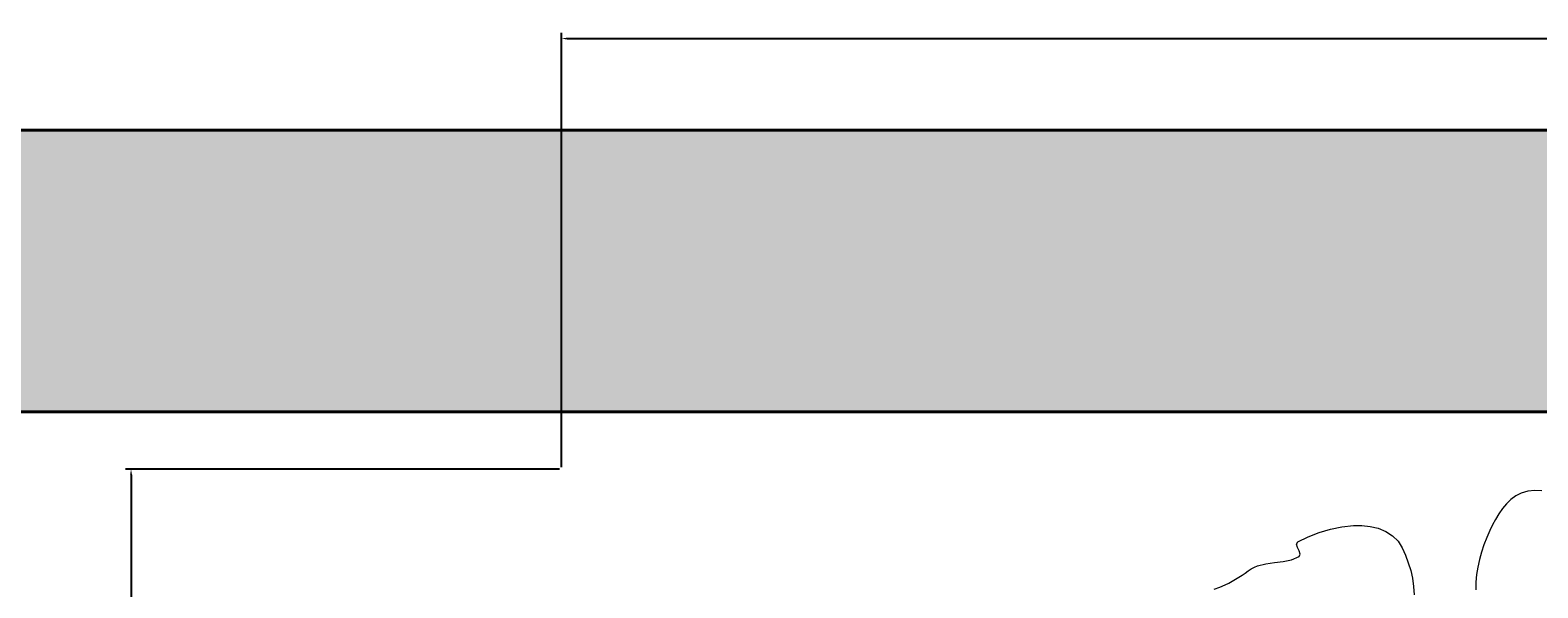
# Model space of a CAD drawing. Units: inches. Extents: x 1441 to 2460, y 1648 to 2683.
# Tile 27 of 35: x 1792 to 1840, y 2284 to 2302. Entities that reach past the tile are written whole.
import ezdxf

# ---------------------------------------------------------------- set-up
doc = ezdxf.new("R2010")
doc.units = ezdxf.units.IN
for name, color, linetype, lineweight in [('A-ANNO-DIMS', 2, 'Continuous', 18), ('A-FURN', 8, 'Continuous', 15), ('A-WALL', 7, 'Continuous', 40)]:
    doc.layers.add(name, color=color, linetype=linetype, lineweight=lineweight)
doc.layers.add('A-WALL-PATT', color=251, linetype='Continuous', lineweight=13, true_color=0x636466)
doc.styles.get("Standard").update_dxf_attribs({"font": 'arial.ttf'})
doc.dimstyles.get("Standard").update_dxf_attribs({"dimtxt": 0.18, "dimasz": 0.18, "dimexe": 0.18, "dimexo": 0.0625, "dimgap": 0.09, "dimtad": 0, "dimtih": 1, "dimtoh": 1, "dimdec": 4, "dimzin": 0, "dimdsep": 46, "dimtxsty": 'Standard', "dimcen": 0.09, "dimadec": 0, "dimazin": 0, "dimtfac": 1, "dimtdec": 4, "dimtofl": 0, "dimtmove": 0, "dimatfit": 3, "dimfxl": 1, "dimtolj": 1, "dimtzin": 0, "dimarcsym": 0})

# ---------------------------------------------------------------- blocks, each defined once
blk = doc.blocks.new('BED-DOUBLE-PLAN')
for p, q in [((30.192, 90.579), (30.063, 90.425)), ((30.333, 90.717), (30.192, 90.579)), ((30.489, 90.832), (30.333, 90.717)), ((30.661, 90.921), (30.489, 90.832)), ((30.874, 90.983), (30.661, 90.921)), ((31.094, 91.001), (30.874, 90.983)), ((31.32, 90.99), (31.094, 91.001)), ((29.842, 90.082), (29.747, 89.903)), ((29.947, 90.257), (29.842, 90.082)), ((30.063, 90.425), (29.947, 90.257)), ((23.852, 89.529), (24.202, 89.666)), ((24.202, 89.666), (24.563, 89.771)), ((24.563, 89.771), (24.931, 89.844)), ((24.931, 89.844), (25.302, 89.885)), ((25.302, 89.885), (25.565, 89.887)), ((25.565, 89.887), (25.831, 89.859)), ((25.831, 89.859), (26.09, 89.797)), ((26.09, 89.797), (26.334, 89.698)), ((26.334, 89.698), (26.554, 89.56)), ((29.66, 89.724), (29.561, 89.501)), ((29.747, 89.903), (29.66, 89.724)), ((23.486, 89.292), (23.52, 89.361)), ((23.516, 89.189), (23.486, 89.292)), ((23.569, 89.075), (23.516, 89.189)), ((23.52, 89.361), (23.852, 89.529)), ((26.554, 89.56), (26.727, 89.384)), ((26.727, 89.384), (26.861, 89.173)), ((26.861, 89.173), (26.965, 88.94)), ((29.471, 89.271), (29.393, 89.037)), ((29.561, 89.501), (29.471, 89.271)), ((22.241, 88.602), (22.507, 88.665)), ((22.507, 88.665), (22.781, 88.701)), ((22.781, 88.701), (23.055, 88.736)), ((23.055, 88.736), (23.32, 88.794)), ((23.32, 88.794), (23.566, 88.9)), ((23.566, 88.9), (23.6, 88.971)), ((23.6, 88.971), (23.569, 89.075)), ((26.965, 88.94), (27.052, 88.696)), ((27.052, 88.696), (27.132, 88.454)), ((29.327, 88.8), (29.274, 88.559)), ((29.393, 89.037), (29.327, 88.8)), ((21.429, 88.107), (21.536, 88.173)), ((21.536, 88.173), (21.643, 88.24)), ((21.643, 88.24), (21.75, 88.305)), ((21.75, 88.305), (21.847, 88.368)), ((21.847, 88.368), (21.942, 88.434)), ((21.942, 88.434), (22.037, 88.5)), ((22.037, 88.5), (22.136, 88.557)), ((22.136, 88.557), (22.241, 88.602)), ((27.132, 88.454), (27.192, 88.199)), ((27.192, 88.199), (27.223, 87.936)), ((29.236, 88.317), (29.214, 88.073)), ((29.274, 88.559), (29.236, 88.317)), ((20.851, 87.851), (21.031, 87.917)), ((21.031, 87.917), (21.207, 87.99)), ((21.207, 87.99), (21.32, 88.045)), ((21.32, 88.045), (21.429, 88.107)), ((27.223, 87.936), (27.246, 87.672)), ((29.214, 88.073), (29.208, 87.829))]:
    blk.add_line(p, q)
blk = doc.blocks.new('*D22')
at = {"layer": 'A-ANNO-DIMS', "color": 0, "lineweight": -2, "transparency": 16777216}
for p, q in [((1809.14, 2287.87), (1795.269, 2287.87)), ((1795.449, 2287.69), (1795.449, 2242.209)), ((1795.449, 2196.362), (1795.449, 2241.843)), ((1809.14, 2196.182), (1795.269, 2196.182))]:
    blk.add_line(p, q, dxfattribs=at)
at = {"layer": 'A-ANNO-DIMS', "color": 0, "transparency": 16777216}
for points in [[(1795.419, 2287.69), (1795.479, 2287.69), (1795.449, 2287.87)], [(1795.419, 2196.362), (1795.479, 2196.362), (1795.449, 2196.182)]]:
    blk.add_solid(points, dxfattribs=at)
at = {"layer": 'Defpoints', "color": 0, "transparency": 16777216}
for p in [(1795.449, 2287.87), (1809.202, 2287.87), (1809.202, 2196.182)]:
    blk.add_point(p, dxfattribs=at)
at = {"layer": 'A-ANNO-DIMS', "color": 0, "transparency": 16777216, "insert": (1795.449, 2242.026), "char_height": 0.18, "attachment_point": 5}
blk.add_mtext('\\A1;DOUBLE BED 92 TYP.', dxfattribs=at)
blk = doc.blocks.new('*D23')
at = {"layer": 'A-ANNO-DIMS', "color": 0, "lineweight": -2, "transparency": 16777216}
for p, q in [((1809.202, 2287.933), (1809.202, 2301.803)), ((1809.382, 2301.623), (1840.924, 2301.623)), ((1873.523, 2301.623), (1841.981, 2301.623)), ((1873.703, 2287.933), (1873.703, 2301.803))]:
    blk.add_line(p, q, dxfattribs=at)
at = {"layer": 'A-ANNO-DIMS', "color": 0, "transparency": 16777216}
for points in [[(1809.382, 2301.653), (1809.382, 2301.593), (1809.202, 2301.623)], [(1873.523, 2301.653), (1873.523, 2301.593), (1873.703, 2301.623)]]:
    blk.add_solid(points, dxfattribs=at)
at = {"layer": 'Defpoints', "color": 0, "transparency": 16777216}
for p in [(1873.703, 2301.623), (1809.202, 2287.87), (1873.703, 2287.87)]:
    blk.add_point(p, dxfattribs=at)
at = {"layer": 'A-ANNO-DIMS', "color": 0, "transparency": 16777216, "insert": (1841.452, 2301.623), "char_height": 0.18, "attachment_point": 5}
blk.add_mtext('\\A1;65 TYP.', dxfattribs=at)
blk = doc.blocks.new('*D67')
at = {"layer": 'A-ANNO-DIMS', "color": 0, "lineweight": -2, "transparency": 16777216}
for p, q in [((1889.448, 2298.695), (1916.216, 2298.695)), ((1916.036, 2298.515), (1916.036, 2055.938)), ((1916.036, 1812.997), (1916.036, 2055.574)), ((1758.224, 1812.817), (1916.216, 1812.817))]:
    blk.add_line(p, q, dxfattribs=at)
at = {"layer": 'A-ANNO-DIMS', "color": 0, "transparency": 16777216}
for points in [[(1916.006, 2298.515), (1916.066, 2298.515), (1916.036, 2298.695)], [(1916.006, 1812.997), (1916.066, 1812.997), (1916.036, 1812.817)]]:
    blk.add_solid(points, dxfattribs=at)
at = {"layer": 'Defpoints', "color": 0, "transparency": 16777216}
for p in [(1889.386, 2298.695), (1916.036, 2298.695), (1758.161, 1812.817)]:
    blk.add_point(p, dxfattribs=at)
at = {"layer": 'A-ANNO-DIMS', "color": 0, "transparency": 16777216, "insert": (1916.036, 2055.756), "char_height": 0.18, "attachment_point": 5}
blk.add_mtext('\\A1;485.9', dxfattribs=at)

msp = doc.modelspace()

# ---------------------------------------------------------------- hatches: boundary and pattern name
at = {"layer": 'A-WALL-PATT'}
h = msp.add_hatch(color=256, dxfattribs=at)
h.dxf.hatch_style = 1
h.paths.add_polyline_path([(1627.5085, 2298.6952), (1568.8859, 2298.6952), (1568.8859, 2246.9605), (1577.8859, 2246.9605), (1577.8859, 2289.6952), (1627.5085, 2289.6952), (1627.5085, 2294.1952)])
h.paths.add_polyline_path([(1675.5777, 2298.6952), (1651.5085, 2298.6952), (1651.5085, 2289.6952), (1675.5777, 2289.6952), (1675.5777, 2294.1952)])
h.paths.add_polyline_path([(1667.3859, 2289.6952), (1662.8859, 2289.6952), (1662.8859, 2233.0622), (1667.3859, 2233.0622)])
h.paths.add_polyline_path([(1715.8721, 2294.3362), (1715.8721, 2295.2788), (1715.8721, 2298.6952), (1699.5777, 2298.6952), (1699.5777, 2289.6952), (1715.8721, 2289.6952)])
h.paths.add_polyline_path([(1707.8859, 2289.6952), (1703.3859, 2289.6952), (1703.3859, 2199.6952), (1707.8859, 2199.6952)])
h.paths.add_polyline_path([(1760.3859, 2204.637), (1755.8859, 2204.637), (1755.8859, 2199.6952), (1667.3859, 2199.6952), (1667.3859, 2204.637), (1662.8859, 2204.637), (1662.8859, 2195.1952), (1760.3859, 2195.1952)])
h.paths.add_polyline_path([(1760.3859, 2289.6952), (1755.8859, 2289.6952), (1755.8859, 2233.0622), (1760.3859, 2233.0622)])
h.paths.add_polyline_path([(1889.3859, 2298.6952), (1739.8721, 2298.6952), (1739.8721, 2289.6952), (1880.3859, 2289.6952), (1880.3859, 2250.8051), (1889.3859, 2250.8051)])
h.paths.add_polyline_path([(1889.3859, 2202.8051), (1880.3859, 2202.8051), (1880.3859, 2157.6952), (1747.948, 2157.6952), (1747.948, 2153.1952), (1755.8859, 2153.1952), (1755.8859, 2058.005), (1760.3859, 2058.005), (1760.3859, 2153.1952), (1880.3859, 2153.1952), (1880.3859, 2124.108), (1889.3859, 2124.108)])
h.paths.add_polyline_path([(1889.3859, 1984.8305), (1880.3859, 1984.8305), (1880.3859, 1834.1952), (1889.3859, 1834.1952)])
h.paths.add_polyline_path([(1889.3859, 2076.108), (1880.3859, 2076.108), (1880.3859, 2008.8305), (1889.3859, 2008.8305)])
h.paths.add_polyline_path([(1880.3859, 2027.1952), (1800.8859, 2027.1952), (1800.8859, 2000.9452), (1805.3859, 2000.9452), (1805.3859, 2022.6952), (1880.3859, 2022.6952)])
h.paths.add_polyline_path([(1800.8859, 2027.1952), (1760.3859, 2027.1952), (1760.3859, 2030.7912), (1755.8859, 2030.7912), (1755.8859, 2022.6952), (1800.8859, 2022.6952)])
h.paths.add_polyline_path([(1880.3859, 1974.6952), (1805.3859, 1974.6952), (1805.3859, 1978.7973), (1800.8859, 1978.7973), (1800.8859, 1974.6952), (1794.8823, 1974.6952), (1794.8823, 1970.1952), (1800.8859, 1970.1952), (1805.3859, 1970.1952), (1880.3859, 1970.1952)])
h.paths.add_polyline_path([(1760.3859, 1974.6952), (1755.8859, 1974.6952), (1755.8859, 1925.6952), (1751.8616, 1925.6952), (1751.8616, 1921.1952), (1760.3859, 1921.1952)])
h.paths.add_polyline_path([(1760.3859, 1921.1952), (1755.8859, 1921.1952), (1755.8859, 1843.1952), (1760.3859, 1843.1952)])
h.paths.add_polyline_path([(1799.1136, 1838.6952), (1799.1136, 1843.1952), (1760.3859, 1843.1952), (1751.8944, 1843.1952), (1751.8944, 1834.1952), (1758.1615, 1834.1952), (1799.1136, 1834.1952)])
h.paths.add_polyline_path([(1880.3859, 1843.1952), (1859.1136, 1843.1952), (1859.1136, 1834.1952), (1880.3859, 1834.1952)])
h.paths.add_polyline_path([(1577.8859, 1857.7914), (1568.8859, 1857.7914), (1568.8859, 1834.1952), (1695.0034, 1834.1952), (1695.0034, 1838.6952), (1695.0034, 1843.1952), (1577.8859, 1843.1952)])
h.paths.add_polyline_path([(1577.8859, 1959.2399), (1573.3859, 1959.2399), (1568.8859, 1959.2399), (1568.8859, 1905.7914), (1577.8859, 1905.7914), (1577.8859, 1921.1952), (1703.3859, 1921.1952), (1707.8859, 1921.1952), (1715.1501, 1921.1952), (1715.1501, 1925.6952), (1707.8859, 1925.6952), (1703.3859, 1925.6952), (1577.8859, 1925.6952)])
h.paths.add_polyline_path([(1577.8859, 2106.6907), (1568.8859, 2106.6907), (1568.8859, 2019.2399), (1577.8859, 2019.2399)])
h.paths.add_polyline_path([(1707.8859, 2051.6952), (1703.3859, 2051.6952), (1703.3859, 2048.6952), (1703.3859, 1925.6952), (1707.8859, 1925.6952)])
h.paths.add_polyline_path([(1703.3859, 2051.6952), (1676.3859, 2051.6952), (1676.3859, 2048.6952), (1703.3859, 2048.6952)])
h.paths.add_polyline_path([(1703.3859, 2102.6952), (1676.3859, 2102.6952), (1676.3859, 2099.6952), (1685.3859, 2099.6952), (1703.3859, 2099.6952)])
h.paths.add_polyline_path([(1707.8859, 2153.1952), (1710.5611, 2153.1952), (1710.5611, 2157.6952), (1707.8859, 2157.6952), (1707.8859, 2195.1952), (1703.3859, 2195.1952), (1703.3859, 2099.6952), (1707.8859, 2099.6952)])
h.paths.add_polyline_path([(1577.8859, 2198.9605), (1568.8859, 2198.9605), (1568.8859, 2166.6907), (1577.8859, 2166.6907)])

# ---------------------------------------------------------------- linework, layer by layer
at = {"layer": 'A-WALL'}
for p, q in [((1568.8859, 2298.6952), (1889.3859, 2298.6952)), ((1577.8859, 2289.6952), (1880.3859, 2289.6952))]:
    msp.add_line(p, q, dxfattribs=at)

# ---------------------------------------------------------------- block references
at = {"layer": 'A-FURN'}
msp.add_blockref('BED-DOUBLE-PLAN', (1809.2, 2196.18), dxfattribs=at)

# ---------------------------------------------------------------- dimensions: what is measured, and where the dimension line sits
at = {"layer": 'A-ANNO-DIMS'}
dim = msp.add_linear_dim(base=(1873.7028, 2301.6233), p1=(1809.2021, 2287.8701), p2=(1873.7028, 2287.8701), text='<> TYP.', dimstyle='Standard', override={"dimdec": 0, "dimlfac": 1, "dimrnd": 0, "dimzin": 0, "dimdsep": 46, "dimlunit": 2}, dxfattribs=at)
dim.commit()
dim.dimension.update_dxf_attribs({"geometry": '*D23', "text_midpoint": (1841.4525, 2301.6233)})
dim = msp.add_linear_dim(base=(1916.0359, 2298.6952), p1=(1758.1615, 1812.8171), p2=(1889.3859, 2298.6952), angle=90, dimstyle='Standard', override={"dimdec": 1, "dimlfac": 1, "dimrnd": 0, "dimzin": 0, "dimdsep": 46, "dimlunit": 2}, dxfattribs=at)
dim.commit()
dim.dimension.update_dxf_attribs({"geometry": '*D67', "text_midpoint": (1916.0359, 2055.7561)})
dim = msp.add_linear_dim(base=(1795.4489, 2287.8701), p1=(1809.2021, 2196.1822), p2=(1809.2021, 2287.8701), angle=90, text='DOUBLE BED <> TYP.', dimstyle='Standard', override={"dimdec": 0, "dimlfac": 1, "dimrnd": 0, "dimzin": 0, "dimdsep": 46, "dimlunit": 2}, dxfattribs=at)
dim.commit()
dim.dimension.update_dxf_attribs({"geometry": '*D22', "text_midpoint": (1795.4489, 2242.0262)})

doc.saveas('drawing.dxf')
